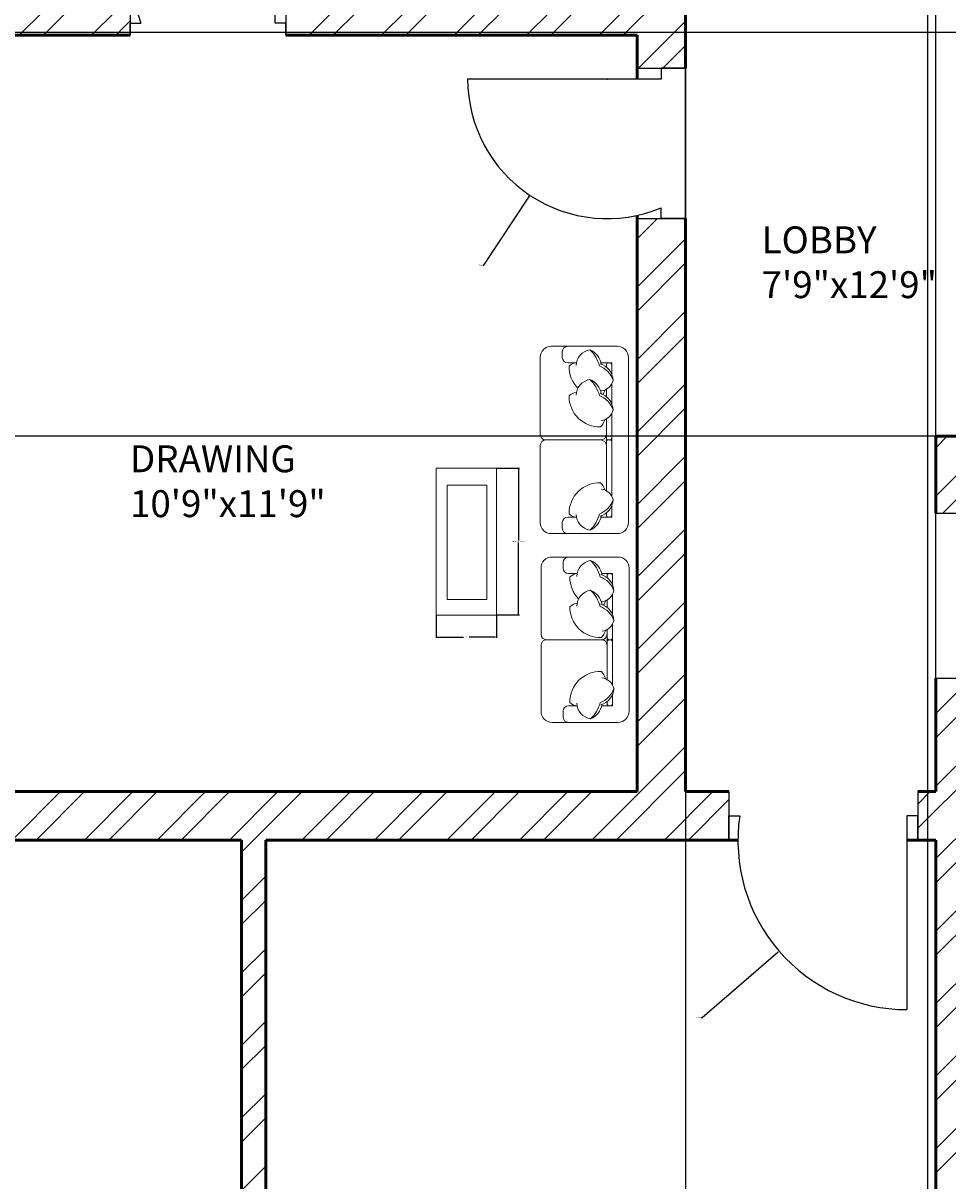
# Model space of a CAD drawing. Units: inches. Extents: x 1896 to 2572, y 1528 to 2474.
# Tile 3 of 10: x 2085 to 2257, y 1818 to 2033. Entities that reach past the tile are written whole.
import ezdxf

# ---------------------------------------------------------------- set-up
doc = ezdxf.new("R2010")
doc.units = ezdxf.units.IN
for name, color, linetype, lineweight in [('A-ANNO-DIMS', 2, 'Continuous', 18), ('A-AREA-IDEN', 7, 'Continuous', 18), ('A-DOOR', 11, 'Continuous', 25), ('A-FURN', 8, 'Continuous', 18), ('A-WALL', 7, 'Continuous', 50)]:
    doc.layers.add(name, color=color, linetype=linetype, lineweight=lineweight)
doc.layers.add('A-WALL-PATT', color=215, linetype='Continuous', lineweight=13, true_color=0xa953a0)
doc.styles.get("Standard").update_dxf_attribs({"font": 'arial.ttf'})
doc.dimstyles.get("Standard").update_dxf_attribs({"dimtxt": 0.18, "dimasz": 0.18, "dimexe": 0.18, "dimexo": 0.0625, "dimgap": 0.09, "dimtad": 0, "dimtih": 1, "dimtoh": 1, "dimdec": 4, "dimzin": 0, "dimdsep": 46, "dimtxsty": 'Standard', "dimcen": 0.09, "dimadec": 0, "dimazin": 0, "dimtfac": 1, "dimtdec": 4, "dimtofl": 0, "dimtmove": 0, "dimatfit": 3, "dimfxl": 1, "dimtolj": 1, "dimtzin": 0, "dimarcsym": 0})

# ---------------------------------------------------------------- blocks, each defined once
blk = doc.blocks.new('TABLE-COFFEE')
for points in [[(11.21, 0), (0, 0), (0, 27.27), (11.21, 27.27)], [(9.42, 2.87), (2.04, 2.87), (2.04, 24.13), (9.42, 24.13)]]:
    blk.add_lwpolyline(points, close=True)
blk = doc.blocks.new('*D13')
at = {"layer": 'A-ANNO-DIMS', "color": 0, "lineweight": -2, "transparency": 16777216}
for p, q in [((2173.04, 1949.97), (2177.25, 1949.97)), ((2177.07, 1949.79), (2177.07, 1936.52)), ((2177.07, 1922.89), (2177.07, 1936.16)), ((2173.04, 1922.71), (2177.25, 1922.71))]:
    blk.add_line(p, q, dxfattribs=at)
at = {"layer": 'A-ANNO-DIMS', "color": 0, "transparency": 16777216}
for points in [[(2177.04, 1949.79), (2177.1, 1949.79), (2177.07, 1949.97)], [(2177.04, 1922.89), (2177.1, 1922.89), (2177.07, 1922.71)]]:
    blk.add_solid(points, dxfattribs=at)
at = {"layer": 'Defpoints', "color": 0, "transparency": 16777216}
for p in [(2172.98, 1949.97), (2177.07, 1949.97), (2172.98, 1922.71)]:
    blk.add_point(p, dxfattribs=at)
at = {"layer": 'A-ANNO-DIMS', "color": 0, "transparency": 16777216, "insert": (2177.07, 1936.34), "char_height": 0.18, "attachment_point": 5}
blk.add_mtext('\\A1;COFFEE TABLE 27 TYP.', dxfattribs=at)
blk = doc.blocks.new('*D14')
at = {"layer": 'A-ANNO-DIMS', "color": 0, "lineweight": -2, "transparency": 16777216}
for p, q in [((2161.77, 1922.65), (2161.77, 1918.44)), ((2172.98, 1922.65), (2172.98, 1918.44)), ((2161.95, 1918.62), (2166.85, 1918.62)), ((2172.8, 1918.62), (2167.89, 1918.62))]:
    blk.add_line(p, q, dxfattribs=at)
at = {"layer": 'A-ANNO-DIMS', "color": 0, "transparency": 16777216}
for points in [[(2161.95, 1918.65), (2161.95, 1918.59), (2161.77, 1918.62)], [(2172.8, 1918.65), (2172.8, 1918.59), (2172.98, 1918.62)]]:
    blk.add_solid(points, dxfattribs=at)
at = {"layer": 'Defpoints', "color": 0, "transparency": 16777216}
for p in [(2161.77, 1922.71), (2172.98, 1922.71), (2172.98, 1918.62)]:
    blk.add_point(p, dxfattribs=at)
at = {"layer": 'A-ANNO-DIMS', "color": 0, "transparency": 16777216, "insert": (2167.37, 1918.62), "char_height": 0.18, "attachment_point": 5}
blk.add_mtext('\\A1;11 TYP.', dxfattribs=at)
blk = doc.blocks.new('*D20')
at = {"layer": 'A-ANNO-DIMS', "color": 0, "lineweight": -2, "transparency": 16777216}
for p, q in [((2180.68, 2431.4), (2511.65, 2431.4)), ((2511.47, 2431.22), (2511.47, 2049.83)), ((2511.47, 1668.08), (2511.47, 2049.47)), ((2452.68, 1667.9), (2511.65, 1667.9))]:
    blk.add_line(p, q, dxfattribs=at)
at = {"layer": 'A-ANNO-DIMS', "color": 0, "transparency": 16777216}
for points in [[(2511.44, 2431.22), (2511.5, 2431.22), (2511.47, 2431.4)], [(2511.44, 1668.08), (2511.5, 1668.08), (2511.47, 1667.9)]]:
    blk.add_solid(points, dxfattribs=at)
at = {"layer": 'Defpoints', "color": 0, "transparency": 16777216}
for p in [(2180.62, 2431.4), (2511.47, 2431.4), (2452.62, 1667.9)]:
    blk.add_point(p, dxfattribs=at)
at = {"layer": 'A-ANNO-DIMS', "color": 0, "transparency": 16777216, "insert": (2511.47, 2049.65), "char_height": 0.18, "attachment_point": 5}
blk.add_mtext('\\A1;763.5', dxfattribs=at)
blk = doc.blocks.new('*D31')
at = {"layer": 'A-ANNO-DIMS', "color": 0, "lineweight": -2, "transparency": 16777216}
for p, q in [((2301.2, 2030.9), (1919.59, 2030.9)), ((1919.77, 2030.72), (1919.77, 1993.58)), ((1919.77, 1956.08), (1919.77, 1993.22)), ((2301.2, 1955.9), (1919.59, 1955.9))]:
    blk.add_line(p, q, dxfattribs=at)
at = {"layer": 'A-ANNO-DIMS', "color": 0, "transparency": 16777216}
for points in [[(1919.74, 2030.72), (1919.8, 2030.72), (1919.77, 2030.9)], [(1919.74, 1956.08), (1919.8, 1956.08), (1919.77, 1955.9)]]:
    blk.add_solid(points, dxfattribs=at)
at = {"layer": 'Defpoints', "color": 0, "transparency": 16777216}
for p in [(1919.77, 2030.9), (2301.26, 2030.9), (2301.26, 1955.9)]:
    blk.add_point(p, dxfattribs=at)
at = {"layer": 'A-ANNO-DIMS', "color": 0, "transparency": 16777216, "insert": (1919.77, 1993.4), "char_height": 0.18, "attachment_point": 5}
blk.add_mtext('\\A1;75', dxfattribs=at)
blk = doc.blocks.new('*D33')
at = {"layer": 'A-ANNO-DIMS', "color": 0, "lineweight": -2, "transparency": 16777216}
for p, q in [((2208.12, 2166.84), (2208.12, 1549.1)), ((2253.12, 2166.84), (2253.12, 1549.1)), ((2208.3, 1549.28), (2230.4, 1549.28)), ((2252.94, 1549.28), (2230.85, 1549.28))]:
    blk.add_line(p, q, dxfattribs=at)
at = {"layer": 'A-ANNO-DIMS', "color": 0, "transparency": 16777216}
for points in [[(2208.3, 1549.31), (2208.3, 1549.25), (2208.12, 1549.28)], [(2252.94, 1549.31), (2252.94, 1549.25), (2253.12, 1549.28)]]:
    blk.add_solid(points, dxfattribs=at)
at = {"layer": 'Defpoints', "color": 0, "transparency": 16777216}
for p in [(2208.12, 2166.9), (2253.12, 2166.9), (2253.12, 1549.28)]:
    blk.add_point(p, dxfattribs=at)
at = {"layer": 'A-ANNO-DIMS', "color": 0, "transparency": 16777216, "insert": (2230.62, 1549.28), "char_height": 0.18, "attachment_point": 5}
blk.add_mtext('\\A1;45', dxfattribs=at)
blk = doc.blocks.new('*D34')
at = {"layer": 'A-ANNO-DIMS', "color": 0, "lineweight": -2, "transparency": 16777216}
for p, q in [((2208.12, 1889.96), (2208.12, 2473.93)), ((2208.3, 2473.75), (2231.04, 2473.75)), ((2254.44, 2473.75), (2231.7, 2473.75)), ((2254.62, 1889.96), (2254.62, 2473.93))]:
    blk.add_line(p, q, dxfattribs=at)
at = {"layer": 'A-ANNO-DIMS', "color": 0, "transparency": 16777216}
for points in [[(2208.3, 2473.78), (2208.3, 2473.72), (2208.12, 2473.75)], [(2254.44, 2473.78), (2254.44, 2473.72), (2254.62, 2473.75)]]:
    blk.add_solid(points, dxfattribs=at)
at = {"layer": 'Defpoints', "color": 0, "transparency": 16777216}
for p in [(2254.62, 2473.75), (2208.12, 1889.9), (2254.62, 1889.9)]:
    blk.add_point(p, dxfattribs=at)
at = {"layer": 'A-ANNO-DIMS', "color": 0, "transparency": 16777216, "insert": (2231.37, 2473.75), "char_height": 0.18, "attachment_point": 5}
blk.add_mtext('\\A1;46.5', dxfattribs=at)
blk = doc.blocks.new('*D36')
at = {"layer": 'A-ANNO-DIMS', "color": 0, "lineweight": -2, "transparency": 16777216}
for p, q in [((2249.19, 1880.82), (2249.37, 1880.82)), ((2249.28, 1880.73), (2249.28, 1880.91)), ((2211.23, 1847.96), (2225.36, 1860.17)), ((2211.05, 1847.96), (2211.23, 1847.96))]:
    blk.add_line(p, q, dxfattribs=at)
at = {"layer": 'A-ANNO-DIMS', "color": 0, "transparency": 16777216}
blk.add_solid([(2225.34, 1860.19), (2225.38, 1860.14), (2225.5, 1860.28)], dxfattribs=at)
at = {"layer": 'Defpoints', "color": 0, "transparency": 16777216}
for p in [(2249.28, 1880.82), (2225.5, 1860.28)]:
    blk.add_point(p, dxfattribs=at)
at = {"layer": 'A-ANNO-DIMS', "color": 0, "transparency": 16777216, "insert": (2210.57, 1847.96), "char_height": 0.18, "attachment_point": 5}
blk.add_mtext('\\A1;R31.42', dxfattribs=at)
blk = doc.blocks.new('*D44')
at = {"layer": 'A-ANNO-DIMS', "color": 0, "lineweight": -2, "transparency": 16777216}
for p, q in [((2193.46, 2022.27), (2193.64, 2022.27)), ((2193.55, 2022.18), (2193.55, 2022.36)), ((2170.61, 1987.7), (2179.11, 2000.51)), ((2170.43, 1987.7), (2170.61, 1987.7))]:
    blk.add_line(p, q, dxfattribs=at)
at = {"layer": 'A-ANNO-DIMS', "color": 0, "transparency": 16777216}
blk.add_solid([(2179.09, 2000.53), (2179.14, 2000.5), (2179.21, 2000.66)], dxfattribs=at)
at = {"layer": 'Defpoints', "color": 0, "transparency": 16777216}
for p in [(2193.55, 2022.27), (2179.21, 2000.66)]:
    blk.add_point(p, dxfattribs=at)
at = {"layer": 'A-ANNO-DIMS', "color": 0, "transparency": 16777216, "insert": (2169.95, 1987.7), "char_height": 0.18, "attachment_point": 5}
blk.add_mtext('\\A1;R25.93', dxfattribs=at)

msp = doc.modelspace()

# ---------------------------------------------------------------- hatches: boundary and pattern name
at = {"layer": 'A-WALL-PATT'}
h = msp.add_hatch(dxfattribs=at)
h.set_pattern_fill('ANSI32', color=256)
h.paths.add_polyline_path([(2071.6224, 2382.3979), (2071.6224, 2422.3979), (2110.6224, 2422.3979), (2110.6224, 2382.3979), (2110.6224, 2357.5961), (2119.6224, 2357.5961), (2119.6224, 2422.3979), (2171.6224, 2422.3979), (2171.6224, 2373.3979), (2193.5093, 2373.3979), (2193.5093, 2377.8979), (2193.5093, 2382.3979), (2180.6224, 2382.3979), (2180.6224, 2431.3979), (2171.6224, 2431.3979), (2119.6224, 2431.3979), (2110.6224, 2431.3979), (2062.6224, 2431.3979), (2062.6224, 2422.3979), (2062.6224, 2382.3979), (1978.6224, 2382.3979), (1978.6224, 2313.0337), (1987.6224, 2313.0337), (1987.6224, 2373.3979), (2062.6224, 2373.3979), (2067.1224, 2373.3979), (2067.1224, 2353.7982), (2071.6224, 2353.8883)])
h.paths.add_polyline_path([(2287.4624, 2382.3979), (2229.5093, 2382.3979), (2229.5093, 2373.3979), (2253.1224, 2373.3979), (2253.1224, 2175.8979), (2247.1039, 2175.8979), (2247.1039, 2166.8979), (2253.1224, 2166.8979), (2253.1224, 2150.8283), (2262.1224, 2150.8283), (2262.1224, 2166.8979), (2262.1224, 2236.8979), (2349.0731, 2236.8979), (2349.0731, 2239.1479), (2349.0731, 2241.3979), (2262.1224, 2241.3979), (2262.1224, 2373.3979), (2287.4624, 2373.3979)])
h.paths.add_polyline_path([(2452.6224, 2382.3979), (2347.4624, 2382.3979), (2347.4624, 2373.3979), (2382.1224, 2373.3979), (2382.1224, 2334.0335), (2386.6224, 2334.0335), (2386.6224, 2373.3979), (2443.6224, 2373.3979), (2443.6224, 2316.2056), (2452.6224, 2316.2056)])
h.paths.add_polyline_path([(2452.6224, 2292.2056), (2448.1224, 2292.2056), (2443.6224, 2292.2056), (2443.6224, 2292.0047), (2443.6224, 2280.9372), (2443.6224, 2268.3979), (2386.6224, 2268.3979), (2386.6224, 2312.4044), (2384.3724, 2312.4044), (2382.1224, 2312.4044), (2382.1224, 2241.3979), (2379.1336, 2241.3979), (2379.1336, 2236.8979), (2386.6224, 2236.8979), (2386.6224, 2263.8979), (2443.6224, 2263.8979), (2443.6224, 2248.8449), (2452.6224, 2248.8449)])
h.paths.add_polyline_path([(2364.1285, 2116.8979), (2262.1224, 2116.8979), (2262.1224, 2120.5401), (2257.6224, 2120.5401), (2253.1224, 2120.5401), (2253.1224, 2107.8979), (2262.1224, 2107.8979), (2269.354, 2107.8979), (2269.354, 2094.0702), (2278.354, 2094.0702), (2278.354, 2107.8979), (2347.6224, 2107.8979), (2347.6224, 2039.8979), (2278.354, 2039.8979), (2278.354, 2054.7605), (2269.354, 2054.7605), (2269.354, 2030.8979), (2278.354, 2030.8979), (2443.6224, 2030.8979), (2443.6224, 2015.198), (2452.6224, 2015.198), (2452.6224, 2030.8979), (2464.6224, 2030.8979), (2469.1224, 2030.8979), (2469.1224, 2117.0352), (2452.6767, 2116.9466), (2452.6285, 2125.8979), (2452.6224, 2125.8979), (2452.6224, 2212.8449), (2443.6224, 2212.8449), (2443.6224, 2116.8979), (2385.832, 2116.8979), (2385.832, 2112.3979), (2385.832, 2107.8979), (2464.6224, 2107.8979), (2464.6224, 2039.8979), (2443.6224, 2039.8979), (2356.6224, 2039.8979), (2356.6224, 2107.8979), (2364.1285, 2107.8979)])
h.paths.add_polyline_path([(2452.6224, 1967.198), (2443.6224, 1967.198), (2443.6224, 1955.8979), (2259.1224, 1955.8979), (2254.6224, 1955.8979), (2254.6224, 1941.6358), (2263.6224, 1941.6358), (2263.6224, 1946.8979), (2379.1224, 1946.8979), (2379.1224, 1913.0204), (2383.6224, 1913.0204), (2383.6224, 1946.8979), (2443.6224, 1946.8979), (2443.6224, 1930.729), (2452.6224, 1930.729)])
h.paths.add_polyline_path([(2469.1224, 1871.8979), (2464.6224, 1871.8979), (2452.6224, 1871.8979), (2452.6224, 1894.729), (2443.6224, 1894.729), (2443.6224, 1871.8979), (2388.1304, 1871.8979), (2388.1304, 1867.3979), (2443.6224, 1867.3979), (2464.6224, 1867.3979), (2464.6224, 1817.8979), (2443.6224, 1817.8979), (2388.1304, 1817.8979), (2388.1304, 1815.6479), (2388.1304, 1813.3979), (2391.1224, 1813.3979), (2391.1224, 1747.8899), (2395.6224, 1747.8899), (2395.6224, 1813.3979), (2443.6224, 1813.3979), (2443.6224, 1781.4434), (2452.6224, 1781.4434), (2452.6224, 1813.3979), (2464.6224, 1813.3979), (2469.1224, 1813.3979)])
h.paths.add_polyline_path([(2263.6224, 1910.9737), (2259.1224, 1910.9737), (2254.6224, 1910.9737), (2254.6224, 1889.8979), (2251.2778, 1889.8979), (2251.2778, 1880.8979), (2254.6224, 1880.8979), (2254.6224, 1817.8979), (2254.6224, 1754.8979), (2254.6224, 1693.3979), (2254.6224, 1684.3979), (2254.6224, 1672.3979), (2200.6224, 1672.3979), (2200.6224, 1684.3979), (2200.6224, 1693.3979), (2200.6224, 1754.8979), (2196.1224, 1754.8979), (2196.1224, 1693.3979), (2150.0488, 1693.3979), (2150.0488, 1684.3979), (2196.1224, 1684.3979), (2196.1224, 1672.3979), (2196.1224, 1667.8979), (2254.6224, 1667.8979), (2259.1224, 1667.8979), (2259.1224, 1693.3979), (2259.1224, 1813.3979), (2353.6224, 1813.3979), (2353.6224, 1815.6479), (2353.6224, 1817.8979), (2263.6224, 1817.8979)])
h.paths.add_polyline_path([(2391.1224, 1693.3979), (2345.6981, 1693.3979), (2345.6981, 1684.3979), (2391.1224, 1684.3979)])
h.paths.add_polyline_path([(2285.6981, 1693.3979), (2259.1224, 1693.3979), (2259.1224, 1684.3979), (2285.6981, 1684.3979), (2285.6981, 1688.8979)], flags=17)
h.paths.add_polyline_path([(2452.6224, 1757.4434), (2448.1224, 1757.4434), (2443.6224, 1757.4434), (2443.6224, 1726.3979), (2395.6224, 1726.3979), (2395.6224, 1728.6572), (2393.3724, 1728.6572), (2391.1224, 1728.6572), (2391.1224, 1717.6723), (2395.6224, 1717.6723), (2395.6224, 1721.8979), (2443.6224, 1721.8979), (2443.6224, 1714.8), (2452.6224, 1714.8)])
h.paths.add_polyline_path([(2452.6224, 1684.3979), (2452.6224, 1690.8), (2443.6224, 1690.8), (2443.6224, 1679.8979), (2443.6224, 1672.3979), (2395.6224, 1672.3979), (2395.6224, 1695.6708), (2391.1224, 1695.5986), (2391.1224, 1672.3979), (2391.1224, 1667.8979), (2452.6224, 1667.8979)])
h.paths.add_polyline_path([(1987.6224, 1880.8979), (2068.6224, 1880.8979), (2125.6224, 1880.8979), (2125.6224, 1788.8466), (2130.1224, 1788.8466), (2130.1224, 1880.8979), (2216.1958, 1880.8979), (2216.1958, 1885.3979), (2216.1958, 1889.8979), (2208.1224, 1889.8979), (2208.1224, 1996.3717), (2203.6224, 1996.3717), (2199.1224, 1996.3717), (2199.1224, 1889.8979), (2073.1224, 1889.8979), (2073.1224, 1917.1874), (2068.6224, 1917.1874), (2068.6224, 1889.8979), (1987.6224, 1889.8979), (1987.6224, 1912.4976), (1978.6224, 1912.4976), (1978.6224, 1805.5193), (1987.6224, 1805.5193)])
h.paths.add_polyline_path([(2019.9303, 1754.8979), (1987.6224, 1754.8979), (1966.6224, 1754.8979), (1966.6224, 1801.0193), (1987.6224, 1801.0193), (1987.6224, 1805.5193), (1962.1224, 1805.5193), (1962.1224, 1750.3979), (1966.6224, 1750.3979), (1978.6224, 1750.3979), (1987.6224, 1750.3979), (2019.9303, 1750.3979)])
h.paths.add_polyline_path([(2135.5566, 1754.8979), (2130.1224, 1754.8979), (2130.1224, 1758.052), (2127.8724, 1758.052), (2125.6224, 1758.052), (2125.6224, 1754.8979), (2068.6224, 1754.8979), (2043.2292, 1754.8979), (2043.2292, 1750.3979), (2068.6224, 1750.3979), (2098.6224, 1750.3979), (2098.6224, 1693.3979), (2068.6224, 1693.3979), (1987.6224, 1693.3979), (1987.6224, 1707.3003), (1983.1224, 1707.3003), (1978.6224, 1707.3003), (1978.6224, 1684.3979), (2068.6224, 1684.3979), (2126.0488, 1684.3979), (2126.0488, 1688.8979), (2126.0488, 1693.3979), (2103.1224, 1693.3979), (2103.1224, 1750.3979), (2130.1224, 1750.3979), (2135.5566, 1750.3979)])
h.paths.add_polyline_path([(1987.6224, 1750.3979), (1978.6224, 1750.3979), (1978.6224, 1731.3003), (1987.6224, 1731.3003)], flags=0)
h.paths.add_polyline_path([(1987.6224, 1973.8979), (2068.6224, 1973.8979), (2073.1224, 1973.8979), (2073.1224, 1978.3979), (1971.1224, 1978.3979), (1971.1224, 2030.3979), (1978.6224, 2030.3979), (1987.6224, 2030.3979), (2104.9199, 2030.3979), (2104.9199, 2032.6479), (2104.9199, 2034.8979), (1987.6224, 2034.8979), (1971.1224, 2034.8979), (1971.1224, 2085.8979), (2003.6464, 2085.8979), (2003.6464, 2090.3979), (1987.6224, 2090.3979), (1987.6224, 2166.8979), (2115.1224, 2166.8979), (2137.6224, 2166.8979), (2137.6224, 2114.4229), (2142.1224, 2114.4229), (2142.1224, 2124.8979), (2153.5306, 2124.8979), (2153.5306, 2127.1479), (2153.5306, 2129.3979), (2142.1224, 2129.3979), (2142.1224, 2166.8979), (2199.1224, 2166.8979), (2199.1224, 2129.3979), (2177.5306, 2129.3979), (2177.5306, 2124.8979), (2199.1224, 2124.8979), (2199.1224, 2034.8979), (2142.1224, 2034.8979), (2142.1224, 2091.6671), (2139.8724, 2091.6671), (2137.6224, 2091.6671), (2137.6224, 2034.8979), (2133.8326, 2034.8979), (2133.8326, 2030.3979), (2137.6224, 2030.3979), (2142.1224, 2030.3979), (2199.1224, 2030.3979), (2199.1224, 2024.2654), (2208.1224, 2024.2654), (2208.1224, 2030.3979), (2208.1224, 2166.8979), (2214.5775, 2166.8979), (2214.5775, 2171.3979), (2214.5775, 2175.8979), (2115.1224, 2175.8979), (2115.1224, 2329.9154), (2112.4137, 2329.9154), (2110.6224, 2329.9154), (2110.6224, 2175.8979), (2082.1224, 2175.8979), (2082.1224, 2202.6443), (2079.8724, 2202.6443), (2077.6224, 2202.6443), (2077.6224, 2175.8979), (1987.6224, 2175.8979), (1987.6224, 2191.3531), (1983.1224, 2191.3531), (1978.6224, 2191.3531), (1978.6224, 2090.3979), (1966.6224, 2090.3979), (1966.6224, 2085.8979), (1966.6224, 2030.3979), (1966.6224, 1973.8979), (1978.6224, 1973.8979), (1978.6224, 1948.4976), (1983.1224, 1948.4976), (1987.6224, 1948.4976)])
h.paths.add_polyline_path([(1987.6224, 2253.0337), (1983.1224, 2253.0337), (1978.6224, 2253.0337), (1978.6224, 2215.3531), (1987.6224, 2215.3531), (1987.6224, 2224.8979), (2077.6224, 2224.8979), (2077.6224, 2221.9854), (2082.1224, 2221.9854), (2082.1224, 2229.3979), (1987.6224, 2229.3979)], flags=17)
h.paths.add_polyline_path([(2220.5047, 1978.7278), (2253.7278, 1978.7278), (2253.7278, 1997.3851), (2220.5047, 1997.3851)], flags=9)
h.paths.add_polyline_path([(2303.6746, 2064.9806), (2320.5334, 2064.9806), (2320.5334, 2075.2842), (2303.6746, 2075.2842)], flags=25)

# ---------------------------------------------------------------- linework, layer by layer
at = {"layer": 'A-DOOR'}
for p, q in [((2131.8326, 2032.6479), (2131.8326, 2068.6479)), ((2104.9199, 2034.8979), (2104.9199, 2030.3979)), ((2133.8326, 2034.8979), (2133.8326, 2030.3979)), ((2104.9199, 2030.3979), (2104.9199, 2032.6479)), ((2104.9199, 2032.6479), (2106.9199, 2032.6479)), ((2133.8326, 2032.6479), (2131.8326, 2032.6479)), ((2133.8326, 2030.3979), (2133.8326, 2032.6479)), ((2199.1224, 2024.2654), (2208.1224, 2024.2654)), ((2208.1224, 2024.2654), (2203.6224, 2024.2654)), ((2203.6224, 2024.2654), (2203.6224, 2022.2654)), ((2203.6224, 2022.2654), (2167.6224, 2022.2654)), ((2203.6224, 1996.3717), (2203.6224, 1998.3717)), ((2199.1224, 1996.3717), (2208.1224, 1996.3717)), ((2208.1224, 1996.3717), (2203.6224, 1996.3717)), ((2254.6224, 1941.6358), (2263.6224, 1941.6358)), ((2254.6224, 1910.9737), (2263.6224, 1910.9737)), ((2216.1958, 1889.8979), (2216.1958, 1880.8979)), ((2251.2778, 1889.8979), (2251.2778, 1880.8979)), ((2216.1958, 1880.8979), (2216.1958, 1885.3979)), ((2216.1958, 1885.3979), (2218.1958, 1885.3979)), ((2251.2778, 1885.3979), (2249.2778, 1885.3979)), ((2249.2778, 1885.3979), (2249.2778, 1849.3979)), ((2251.2778, 1880.8979), (2251.2778, 1885.3979))]:
    msp.add_line(p, q, dxfattribs=at)
for centre, radius, start, end in [((2131.8326, 2042.0278), 26.6201, 90, 200.631887), ((2193.5517, 2022.2654), 25.9293, 180, 292.854556), ((2249.2778, 1880.8158), 31.4179, 171.613893, 270)]:
    msp.add_arc(centre, radius, start, end, dxfattribs=at)
at = {"layer": 'A-FURN', "ltscale": 0.03}
for points in [[(2181.1232, 1954.1948, -0.41421356), (2182.1466, 1955.2182, -0.41421356), (2181.1232, 1956.2416), (2181.1232, 1970.5693, -0.41421356), (2183.17, 1972.6161), (2195.4509, 1972.6161, -0.41421356), (2197.4977, 1970.5693), (2197.4977, 1939.8671, -0.41421356), (2195.4509, 1937.8203), (2183.17, 1937.8203, -0.41421356), (2181.1232, 1939.8671), (2181.1232, 1954.1948, -0.41421356), (2182.1466, 1955.2182, -0.41421356), (2181.1232, 1956.2416)], [(2181.2607, 1917.0957, -0.41421356), (2182.2841, 1918.1191, -0.41421356), (2181.2607, 1919.1425), (2181.2607, 1931.4234, -0.41421356), (2183.3075, 1933.4703), (2195.5884, 1933.4703, -0.41421356), (2197.6352, 1931.4234), (2197.6352, 1904.8148, -0.41421356), (2195.5884, 1902.768), (2183.3075, 1902.768, -0.41421356), (2181.2607, 1904.8148), (2181.2607, 1917.0957, -0.41421356), (2182.2841, 1918.1191, -0.41421356), (2181.2607, 1919.1425)]]:
    msp.add_lwpolyline(points, format="xyb", dxfattribs=at)
at = {"layer": 'A-FURN'}
for points in [[(2187.8259, 1969.5459), (2186.2403, 1969.5459, -0.41421356), (2185.2169, 1970.5693), (2185.2169, 1971.5927, -0.41421356), (2186.2403, 1972.6161)], [(2187.764, 1969.0323, -0.35677236), (2190.3436, 1971.9648, -0.24954205), (2192.4694, 1969.3077, 9.61688035)], [(2190.3436, 1971.9648, -0.14772988), (2192.1024, 1968.9737, -0.21334276), (2194.682, 1966.3344, -0.17866181)], [(2187.8264, 1969.5481, 0.16554063), (2186.4741, 1968.915, 0.20023115), (2188.121, 1964.8525, 0.12152332)], [(2192.2426, 1969.3869, -0.30666349), (2194.682, 1966.3344, -0.30632997), (2192.4542, 1964.3403, 0.87284716)], [(2194.4275, 1967.3929), (2194.4275, 1969.5459), (2192.4163, 1969.5459, -0.41421356)], [(2193.4041, 1968.7649), (2193.4041, 1969.1365, -0.41421356), (2193.8135, 1969.5459), (2194.0182, 1969.5459, -0.41421356), (2194.4275, 1969.1365)], [(2194.4275, 1969.1365), (2194.4275, 1967.3929, -0.41421356)], [(2187.764, 1963.5193, -0.35677236), (2190.3436, 1966.4517, -0.24954205), (2192.4694, 1963.7946, 9.61688035)], [(2190.3436, 1966.4517, -0.14772988), (2192.1024, 1963.4606, -0.21334276), (2194.682, 1960.8214, -0.17866181)], [(2194.4275, 1965.6904), (2194.4275, 1961.8799, -0.41421356)], [(2187.8264, 1964.0351, 0.16554063), (2186.4741, 1963.402, 0.42598917), (2192.3369, 1957.6543, 0.12152332), (2193.145, 1959.0187, -7.11546429)], [(2192.2426, 1963.8738, -0.30666349), (2194.682, 1960.8214, -0.30632997), (2192.4542, 1958.8273, 0.87284716)], [(2192.7449, 1963.6737, 0.07186538), (2193.145, 1964.5317, -7.11546429)], [(2193.4041, 1963.2519), (2193.4041, 1964.6598, -0.41421356)], [(2194.4275, 1960.1773), (2194.4275, 1955.6276, -0.41421356), (2194.0182, 1955.2182), (2193.8135, 1955.2182, -0.41421356), (2193.4041, 1955.6276), (2193.4041, 1959.1468, -0.41421356)], [(2193.4041, 1956.2416, -0.41421356), (2192.3807, 1955.2182), (2182.1466, 1955.2182, -0.41421356)], [(2193.4041, 1954.1948, 0.41421356), (2192.3807, 1955.2182), (2182.1466, 1955.2182, 0.41421356)], [(2193.4041, 1956.2416, -0.41421356), (2192.3807, 1955.2182)], [(2193.4041, 1954.1948, 0.41421356), (2192.3807, 1955.2182)], [(2194.4275, 1944.746), (2194.4275, 1954.8088, 0.41421356), (2194.0182, 1955.2182), (2193.8135, 1955.2182, 0.41421356), (2193.4041, 1954.8088), (2193.4041, 1945.7765, 0.41421356)], [(2187.8264, 1940.8883, -0.16554063), (2186.4741, 1941.5214, -0.42598917), (2192.3369, 1947.269, -0.12152332), (2193.145, 1945.9046, 7.11546429)], [(2190.3436, 1938.4716, 0.14772988), (2192.1024, 1941.4627, 0.21334276), (2194.682, 1944.1019, 0.17866181)], [(2192.2426, 1941.0495, 0.30666349), (2194.682, 1944.1019, 0.30632997), (2192.4542, 1946.096, -0.87284716)], [(2194.4275, 1941.2998), (2194.4275, 1943.0434, 0.41421356)], [(2186.2403, 1937.8203, -0.41421356), (2185.2169, 1938.8437), (2185.2169, 1939.8671, -0.41421356), (2186.2403, 1940.8905), (2187.8259, 1940.8905)], [(2187.764, 1941.4041, 0.35677236), (2190.3436, 1938.4716, 0.24954205), (2192.4694, 1941.1287, -9.61688035)], [(2193.4041, 1941.6715), (2193.4041, 1941.2998, 0.41421356), (2193.8135, 1940.8905), (2194.0182, 1940.8905, 0.41421356), (2194.4275, 1941.2998)], [(2187.9634, 1930.4), (2186.3778, 1930.4, -0.41421356), (2185.3543, 1931.4234), (2185.3543, 1932.4468, -0.41421356), (2186.3778, 1933.4703)], [(2187.9014, 1929.8864, -0.35677236), (2190.4811, 1932.8189, -0.24954205), (2192.6069, 1930.1618, 9.61688035)], [(2190.4811, 1932.8189, -0.14772988), (2192.2399, 1929.8278, -0.21334276), (2194.8195, 1927.1886, -0.17866181)], [(2187.9638, 1930.4023, 0.16554063), (2186.6116, 1929.7691, 0.20023115), (2188.2585, 1925.7066, 0.12152332)], [(2192.3801, 1930.241, -0.30666349), (2194.8195, 1927.1886, -0.30632997), (2192.5917, 1925.1945, 0.87284716)], [(2194.565, 1928.2471), (2194.565, 1930.4), (2192.5538, 1930.4, -0.41421356)], [(2193.5416, 1929.619), (2193.5416, 1929.9907, -0.41421356), (2193.951, 1930.4), (2194.1557, 1930.4, -0.41421356), (2194.565, 1929.9907)], [(2194.565, 1929.9907), (2194.565, 1928.2471, -0.41421356)], [(2187.9014, 1924.3734, -0.35677236), (2190.4811, 1927.3059, -0.24954205), (2192.6069, 1924.6488, 9.61688035)], [(2190.4811, 1927.3059, -0.14772988), (2192.2399, 1924.3147, -0.21334276), (2194.8195, 1921.6755, -0.17866181)], [(2187.9638, 1924.8892, 0.16554063), (2186.6116, 1924.2561, 0.42598917), (2192.4744, 1918.5084, 0.12152332), (2193.2825, 1919.8728, -7.11546429)], [(2192.3801, 1924.728, -0.30666349), (2194.8195, 1921.6755, -0.30632997), (2192.5917, 1919.6814, 0.87284716)], [(2192.8824, 1924.5279, 0.07186538), (2193.2825, 1925.3859, -7.11546429)], [(2193.5416, 1924.106), (2193.5416, 1925.514, -0.41421356)], [(2194.565, 1926.5445), (2194.565, 1922.734, -0.41421356)], [(2194.565, 1921.0314), (2194.565, 1918.5285, -0.41421356), (2194.1557, 1918.1191), (2193.951, 1918.1191, -0.41421356), (2193.5416, 1918.5285), (2193.5416, 1920.0009, -0.41421356)], [(2193.5416, 1919.1425, -0.41421356), (2192.5182, 1918.1191), (2182.2841, 1918.1191, -0.41421356)], [(2193.5416, 1919.1425, -0.41421356), (2192.5182, 1918.1191)], [(2193.5416, 1917.0957, 0.41421356), (2192.5182, 1918.1191), (2182.2841, 1918.1191, 0.41421356)], [(2193.5416, 1917.0957, 0.41421356), (2192.5182, 1918.1191)], [(2194.565, 1909.6938), (2194.565, 1917.7098, 0.41421356), (2194.1557, 1918.1191), (2193.951, 1918.1191, 0.41421356), (2193.5416, 1917.7098), (2193.5416, 1910.7243, 0.41421356)], [(2187.9638, 1905.836, -0.16554063), (2186.6116, 1906.4691, -0.42598917), (2192.4744, 1912.2168, -0.12152332), (2193.2825, 1910.8524, 7.11546429)], [(2192.3801, 1905.9972, 0.30666349), (2194.8195, 1909.0497, 0.30632997), (2192.5917, 1911.0438, -0.87284716)], [(2190.4811, 1903.4193, 0.14772988), (2192.2399, 1906.4105, 0.21334276), (2194.8195, 1909.0497, 0.17866181)], [(2194.565, 1906.2476), (2194.565, 1907.9912, 0.41421356)], [(2186.3778, 1902.768, -0.41421356), (2185.3543, 1903.7914), (2185.3543, 1904.8148, -0.41421356), (2186.3778, 1905.8382), (2187.9634, 1905.8382)], [(2187.9014, 1906.3518, 0.35677236), (2190.4811, 1903.4193, 0.24954205), (2192.6069, 1906.0764, -9.61688035)], [(2193.5416, 1906.6192), (2193.5416, 1906.2476, 0.41421356), (2193.951, 1905.8382), (2194.1557, 1905.8382, 0.41421356), (2194.565, 1906.2476)]]:
    msp.add_lwpolyline(points, format="xyb", dxfattribs=at)
for points in [[(2194.4275, 1961.8799), (2194.4275, 1965.6904)], [(2194.4275, 1944.746), (2194.4275, 1960.1773)], [(2192.4163, 1940.8905), (2194.4275, 1940.8905), (2194.4275, 1943.0434)], [(2194.565, 1922.734), (2194.565, 1926.5445)], [(2194.565, 1909.6938), (2194.565, 1921.0314)], [(2192.5538, 1905.8382), (2194.565, 1905.8382), (2194.565, 1907.9912)]]:
    msp.add_lwpolyline(points, dxfattribs=at)
for points in [[(2194.4275, 1954.8088), (2194.4275, 1955.6276, -0.41421356), (2194.0182, 1955.2182), (2193.8135, 1955.2182, -0.41421356), (2193.4041, 1955.6276), (2193.4041, 1954.8088, -0.41421356), (2193.8135, 1955.2182), (2194.0182, 1955.2182, -0.41421356)], [(2194.565, 1917.7098), (2194.565, 1918.5285, -0.41421356), (2194.1557, 1918.1191), (2193.951, 1918.1191, -0.41421356), (2193.5416, 1918.5285), (2193.5416, 1917.7098, -0.41421356), (2193.951, 1918.1191), (2194.1557, 1918.1191, -0.41421356)]]:
    msp.add_lwpolyline(points, format="xyb", close=True, dxfattribs=at)
at = {"layer": 'A-WALL'}
for p, q in [((2208.1224, 2166.8979), (2208.1224, 2030.3979)), ((1987.6224, 2030.3979), (2104.9199, 2030.3979)), ((2133.8326, 2030.3979), (2137.6224, 2030.3979)), ((2137.6224, 2030.3979), (2142.1224, 2030.3979)), ((2142.1224, 2030.3979), (2199.1224, 2030.3979)), ((2199.1224, 2022.2654), (2199.1224, 2030.3979)), ((2208.1224, 2030.3979), (2208.1224, 2024.2654)), ((2199.1224, 1889.8979), (2199.1224, 1996.9416)), ((2208.1224, 1996.3717), (2208.1224, 1889.8979)), ((2254.6224, 1955.8979), (2263.6224, 1955.8979)), ((2254.6224, 1941.6358), (2254.6224, 1955.8979)), ((2254.6224, 1889.8979), (2254.6224, 1910.9737)), ((2199.1224, 1889.8979), (2073.1224, 1889.8979)), ((2216.1958, 1889.8979), (2208.1224, 1889.8979)), ((2254.6224, 1889.8979), (2251.2778, 1889.8979)), ((2068.6224, 1880.8979), (2125.6224, 1880.8979)), ((2125.6224, 1880.8979), (2125.6224, 1787.4201)), ((2130.1224, 1880.8979), (2130.1224, 1788.8466)), ((2130.1224, 1880.8979), (2217.86, 1880.8979)), ((2208.1224, 1880.8979), (2199.1224, 1880.8979)), ((2249.2778, 1880.8979), (2254.6224, 1880.8979)), ((2254.6224, 1817.8979), (2254.6224, 1880.8979)), ((2254.6224, 1817.8979), (2254.6224, 1754.8979))]:
    msp.add_line(p, q, dxfattribs=at)

# ---------------------------------------------------------------- block references
at = {"layer": 'A-FURN'}
msp.add_blockref('TABLE-COFFEE', (2161.769, 1922.708), dxfattribs=at)

# ---------------------------------------------------------------- texts
at = {"layer": 'A-AREA-IDEN', "char_height": 5, "attachment_point": 1}
for s, width, insert in [('LOBBY\\P7\'9"x12\'9"', 114.363402, (2222.2663, 1994.9005)), ('DRAWING\\P10\'9"x11\'9"', 158.737602, (2104.8848, 1954.2236))]:
    msp.add_mtext_dynamic_manual_height_columns(s, width=width, gutter_width=12.5, heights=[0], dxfattribs=dict(at, insert=insert))

# ---------------------------------------------------------------- dimensions: what is measured, and where the dimension line sits
at = {"layer": 'A-ANNO-DIMS'}
for base, p1, p2, override, picture, middle in [((2254.6224, 2473.7479), (2208.1224, 1889.8979), (2254.6224, 1889.8979), {"dimdec": 1, "dimlfac": 1, "dimrnd": 0, "dimzin": 0, "dimdsep": 46, "dimlunit": 2}, '*D34', (2231.3724, 2473.7479)), ((2253.1224, 1549.2803), (2208.1224, 2166.8979), (2253.1224, 2166.8979), {"dimdec": 0, "dimlfac": 1, "dimrnd": 0, "dimzin": 0, "dimdsep": 46, "dimlunit": 2}, '*D33', (2230.6224, 1549.2803))]:
    dim = msp.add_linear_dim(base=base, p1=p1, p2=p2, dimstyle='Standard', override=override, dxfattribs=at)
    dim.commit()
    dim.dimension.update_dxf_attribs({"geometry": picture, "text_midpoint": middle})
for base, p1, p2, override, picture, middle in [((2511.4724, 2431.3979), (2452.6224, 1667.8979), (2180.6224, 2431.3979), {"dimdec": 1, "dimlfac": 1, "dimrnd": 0, "dimzin": 0, "dimdsep": 46, "dimlunit": 2}, '*D20', (2511.4724, 2049.6479)), ((1919.7724, 2030.8979), (2301.2636, 1955.8979), (2301.2636, 2030.8979), {"dimdec": 0, "dimlfac": 1, "dimrnd": 0, "dimzin": 0, "dimdsep": 46, "dimlunit": 2}, '*D31', (1919.7724, 1993.3979))]:
    dim = msp.add_linear_dim(base=base, p1=p1, p2=p2, angle=90, dimstyle='Standard', override=override, dxfattribs=at)
    dim.commit()
    dim.dimension.update_dxf_attribs({"geometry": picture, "text_midpoint": middle})
for center, mpoint, picture, middle in [((2193.5517, 2022.2654), (2179.2128, 2000.6616), '*D44', (2169.9496, 1987.6994)), ((2249.2778, 1880.8158), (2225.4969, 1860.2839), '*D36', (2210.5695, 1847.9648))]:
    dim = msp.add_radius_dim(center=center, mpoint=mpoint, dimstyle='Standard', override={"dimdec": 2, "dimlfac": 1, "dimrnd": 0, "dimzin": 0, "dimdsep": 46, "dimlunit": 2}, dxfattribs=at)
    dim.commit()
    dim.dimension.update_dxf_attribs({"geometry": picture, "text_midpoint": middle, "dimtype": 164})
dim = msp.add_linear_dim(base=(2177.0659, 1949.9749), p1=(2172.9759, 1922.7083), p2=(2172.9759, 1949.9749), angle=90, text='COFFEE TABLE <> TYP.', dimstyle='Standard', override={"dimdec": 0, "dimlfac": 1, "dimrnd": 0, "dimzin": 0, "dimdsep": 46, "dimlunit": 2}, dxfattribs=at)
dim.commit()
dim.dimension.update_dxf_attribs({"geometry": '*D13', "text_midpoint": (2177.0659, 1936.3416)})
dim = msp.add_linear_dim(base=(2172.9759, 1918.6183), p1=(2161.7688, 1922.7083), p2=(2172.9759, 1922.7083), text='<> TYP.', dimstyle='Standard', override={"dimdec": 0, "dimlfac": 1, "dimrnd": 0, "dimzin": 0, "dimdsep": 46, "dimlunit": 2}, dxfattribs=at)
dim.commit()
dim.dimension.update_dxf_attribs({"geometry": '*D14', "text_midpoint": (2167.3724, 1918.6183)})

doc.saveas('drawing.dxf')
